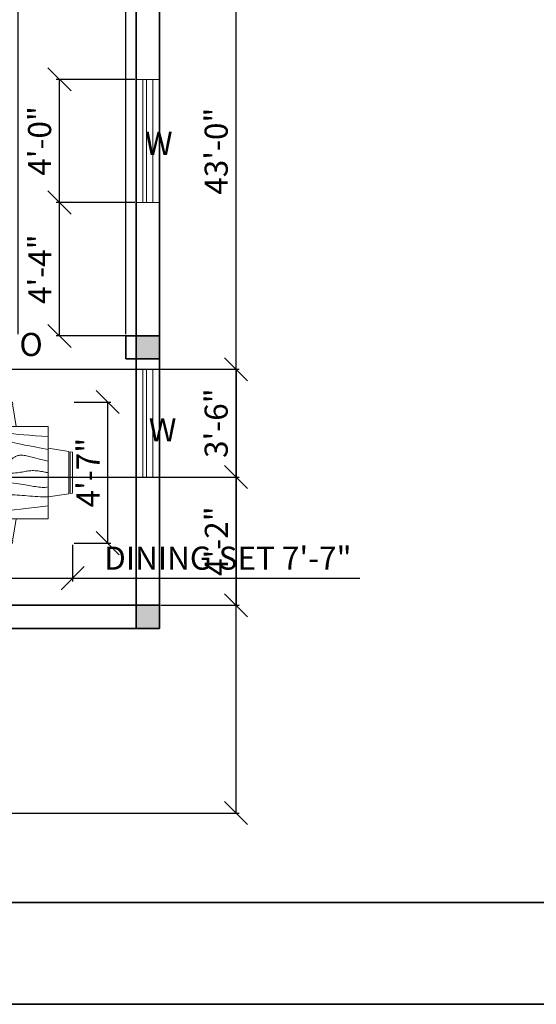
# Model space of a CAD drawing. Units: inches. Extents: x 1798 to 3594, y 1405 to 2404.
# Tile 3 of 6: x 2457 to 2658, y 1405 to 1789. Entities that reach past the tile are written whole.
import ezdxf

# ---------------------------------------------------------------- set-up
doc = ezdxf.new("R2010")
doc.units = ezdxf.units.IN
for name, color, linetype, lineweight in [('A-ANNO-DIMS', 6, 'Continuous', 18), ('A-ANNO-TEXT', 7, 'Continuous', 18), ('A-ANNO-TTLB', 7, 'Continuous', 35), ('A-FURN', 18, 'Continuous', 18), ('A-GLAZ', 4, 'Continuous', 18), ('A-WALL', 7, 'Continuous', 35), ('S-COLS', 1, 'Continuous', 35)]:
    doc.layers.add(name, color=color, linetype=linetype, lineweight=lineweight)
doc.styles.get("Standard").update_dxf_attribs({"font": 'arial.ttf'})
doc.dimstyles.new('ISO-25', dxfattribs={"dimtxt": 9, "dimasz": 9, "dimexe": 1.25, "dimexo": 0.625, "dimgap": 2, "dimtad": 1, "dimdec": 1, "dimlunit": 4, "dimtxsty": 'Standard', "dimblk": 'OBLIQUE', "dimcen": 2.5, "dimazin": 0, "dimtfac": 1, "dimtdec": 1, "dimtmove": 0, "dimatfit": 3, "dimfxl": 1, "dimarcsym": 0})

# ---------------------------------------------------------------- blocks, each defined once
blk = doc.blocks.new('Dining Set - 36 x 72 in.')
for p, q in [((-22, 27.5), (-22.1562, 26.50042)), ((-22, 27.5), (-6, 27.5)), ((-5.8437, 26.49966), (-6, 27.5)), ((6, 27.5), (5.8438, 26.50042)), ((6, 27.5), (22, 27.5)), ((22.1563, 26.49966), (22, 27.5)), ((-22.2343, 26.00059), (-23.4847, 17.99762)), ((-22.2304, 26), (-5.7608, 26)), ((-5.8416, 26.5), (-22.1534, 26.5)), ((-4.5152, 17.99762), (-5.7655, 25.99926)), ((5.7657, 26.00059), (4.5153, 17.99762)), ((5.7696, 26), (22.2392, 26)), ((22.1584, 26.5), (5.8466, 26.5)), ((23.4848, 17.99762), (22.2345, 25.99926)), ((36, 18), (-36, 18)), ((-36, 18), (-36, -18)), ((36, -18), (36, 18)), ((-45.5, 8), (-44.5004, 8.15617)), ((-45.5, 8), (-45.5, -8)), ((-44.5, -8.15843), (-44.5, 8.15338)), ((-44.0006, 8.23428), (-35.9976, 9.48474)), ((-44, 8.23041), (-44, -8.23915)), ((44.0006, 8.23428), (35.9976, 9.48474)), ((44, 8.23041), (44, -8.23915)), ((44.5, -8.15843), (44.5, 8.15338)), ((45.5, 8), (44.5005, 8.15617)), ((45.5, 8), (45.5, -8)), ((-44.4997, -8.15631), (-45.5, -8)), ((-35.9976, -9.48476), (-43.9993, -8.2345)), ((35.9976, -9.48476), (43.9993, -8.2345)), ((44.4997, -8.15631), (45.5, -8)), ((-36, -18), (36, -18)), ((-22.2343, -26.0006), (-23.4847, -17.99762)), ((-4.5152, -17.99762), (-5.7655, -25.99928)), ((5.7657, -26.0006), (4.5153, -17.99762)), ((23.4848, -17.99762), (22.2345, -25.99928)), ((-22.2304, -26), (-5.7608, -26)), ((-22, -27.5), (-22.1562, -26.50044)), ((-5.8416, -26.5), (-22.1534, -26.5)), ((-5.8437, -26.49967), (-6, -27.5)), ((5.7696, -26), (22.2392, -26)), ((6, -27.5), (5.8438, -26.50044)), ((22.1584, -26.5), (5.8466, -26.5)), ((22.1563, -26.49967), (22, -27.5)), ((-22, -27.5), (-6, -27.5)), ((6, -27.5), (22, -27.5))]:
    blk.add_line(p, q)
for points in [[(-36, 15), (-31.1772, 14.97754), (-26.8079, 14.91406), (-22.8538, 14.81543), (-19.276, 14.6875), (-16.0362, 14.53613), (-13.0957, 14.36718), (-10.4159, 14.18652), (-7.9583, 14), (-5.6904, 13.81315), (-3.6035, 13.63021), (-1.6954, 13.45508), (0.0365, 13.29166), (1.5945, 13.14388), (2.9811, 13.01562), (4.1988, 12.9108), (5.25, 12.83333), (6.1393, 12.78613), (6.8802, 12.76823), (7.4883, 12.77767), (7.9792, 12.8125), (8.3685, 12.87077), (8.6719, 12.95052), (8.9049, 13.0498), (9.0833, 13.16666), (9.2205, 13.29899), (9.3216, 13.44401), (9.3895, 13.59879), (9.4271, 13.76041), (9.4373, 13.92594), (9.4232, 14.09245), (9.3875, 14.257), (9.3333, 14.41666), (9.2638, 14.56917), (9.1836, 14.71484), (9.0975, 14.85465), (9.0104, 14.98958), (8.9272, 15.1206), (8.8529, 15.2487), (8.7922, 15.37483), (8.75, 15.5), (8.7305, 15.62467), (8.7344, 15.74739), (8.7617, 15.86621), (8.8125, 15.97916), (8.8867, 16.08431), (8.9844, 16.17968), (9.1055, 16.26334), (9.25, 16.33333), (9.4189, 16.38802), (9.6172, 16.42708), (9.8506, 16.45052), (10.125, 16.45833), (10.4463, 16.45052), (10.8203, 16.42708), (11.2529, 16.38802), (11.75, 16.33333), (12.3184, 16.26318), (12.9694, 16.17838), (13.7151, 16.07991), (14.5677, 15.96875), (15.5395, 15.84586), (16.6426, 15.71224), (17.8893, 15.56884), (19.2917, 15.41666), (20.859, 15.25667), (22.5879, 15.08984), (24.4721, 14.91715), (26.5052, 14.73958), (28.6809, 14.5581), (30.9929, 14.3737), (33.4347, 14.18733), (36, 14)], [(-36, 10), (-28.9766, 10.14274), (-23.1725, 10.20442), (-18.4241, 10.19775), (-14.5677, 10.13541), (-11.4399, 10.03011), (-8.877, 9.89453), (-6.7154, 9.74137), (-4.7917, 9.58333), (-2.9698, 9.43082), (-1.2246, 9.28515), (0.4415, 9.14534), (2.026, 9.01041), (3.5266, 8.87939), (4.9408, 8.7513), (6.266, 8.62516), (7.5, 8.5), (8.6411, 8.37549), (9.6914, 8.2539), (10.6538, 8.13818), (11.5312, 8.03125), (12.3267, 7.93603), (13.043, 7.85547), (13.6831, 7.79248), (14.25, 7.75), (14.7471, 7.7303), (15.1797, 7.73307), (15.5537, 7.75732), (15.875, 7.80208), (16.1494, 7.86637), (16.3828, 7.94922), (16.5811, 8.04964), (16.75, 8.16666), (16.8944, 8.29915), (17.0143, 8.44531), (17.1089, 8.60319), (17.1771, 8.77083), (17.218, 8.94629), (17.2305, 9.1276), (17.2137, 9.31282), (17.1667, 9.5), (17.0895, 9.6875), (16.987, 9.875), (16.8649, 10.0625), (16.7292, 10.25), (16.5856, 10.4375), (16.4401, 10.625), (16.2985, 10.8125), (16.1667, 11), (16.05, 11.18733), (15.9518, 11.3737), (15.8752, 11.5581), (15.8229, 11.73958), (15.798, 11.91715), (15.8034, 12.08984), (15.842, 12.25667), (15.9167, 12.41666), (16.0295, 12.56836), (16.1784, 12.70833), (16.3605, 12.83268), (16.5729, 12.9375), (16.8127, 13.01888), (17.0768, 13.07291), (17.3625, 13.0957), (17.6667, 13.08333), (17.9894, 13.03312), (18.3418, 12.94726), (18.7382, 12.82918), (19.1927, 12.68229), (19.7195, 12.51001), (20.3327, 12.31575), (21.0465, 12.10294), (21.875, 11.875), (22.8357, 11.63354), (23.959, 11.37304), (25.2786, 11.08618), (26.8282, 10.76562), (28.6414, 10.40405), (30.752, 9.99414), (33.1936, 9.52856), (36, 9)], [(-36, 5.5), (-30.7157, 5.3348), (-26.069, 5.20963), (-21.9946, 5.11767), (-18.4271, 5.05208), (-15.3009, 5.00602), (-12.5508, 4.97265), (-10.1112, 4.94515), (-7.9167, 4.91666), (-5.909, 4.88167), (-4.0586, 4.83984), (-2.3429, 4.79215), (-0.7396, 4.73958), (0.7739, 4.6831), (2.22, 4.6237), (3.6213, 4.56233), (5, 4.5), (6.373, 4.43782), (7.7344, 4.3776), (9.0723, 4.32129), (10.375, 4.27083), (11.6309, 4.22819), (12.8281, 4.19531), (13.9551, 4.17415), (15, 4.16666), (15.954, 4.17448), (16.819, 4.19791), (17.6001, 4.23698), (18.3021, 4.29166), (18.9299, 4.36198), (19.4883, 4.44791), (19.9823, 4.54948), (20.4167, 4.66666), (20.7969, 4.79899), (21.1302, 4.94401), (21.4245, 5.09879), (21.6875, 5.26041), (21.9271, 5.42594), (22.1511, 5.59245), (22.3672, 5.757), (22.5834, 5.91666), (22.8065, 6.06868), (23.0404, 6.21093), (23.2879, 6.34147), (23.5521, 6.45833), (23.8358, 6.55957), (24.142, 6.64323), (24.4735, 6.70735), (24.8334, 6.75), (25.2235, 6.76969), (25.642, 6.76692), (26.0858, 6.74267), (26.5521, 6.69791), (27.0379, 6.63362), (27.5404, 6.55078), (28.0565, 6.45036), (28.5834, 6.33333), (29.1242, 6.19987), (29.7071, 6.04687), (30.3661, 5.87044), (31.1354, 5.66666), (32.0493, 5.43164), (33.142, 5.16146), (34.4475, 4.85221), (36, 4.5)], [(-36, -1), (-30.7915, -0.6591), (-26.0195, -0.38216), (-21.6519, -0.16284), (-17.6563, 0.00521), (-14.0005, 0.12833), (-10.6523, 0.21289), (-7.5796, 0.26522), (-4.75, 0.29166), (-2.134, 0.29793), (0.2878, 0.28711), (2.5317, 0.26163), (4.6146, 0.22396), (6.5529, 0.17651), (8.3633, 0.12174), (10.0623, 0.06209), (11.6667, 0), (13.1899, -0.06201), (14.6341, -0.1211), (15.9982, -0.17432), (17.2813, -0.21875), (18.4823, -0.25147), (19.6003, -0.26953), (20.6343, -0.27002), (21.5834, -0.25), (22.4481, -0.20768), (23.2357, -0.14584), (23.9549, -0.06836), (24.6146, 0.02083), (25.2235, 0.11784), (25.7904, 0.21875), (26.3241, 0.31966), (26.8334, 0.41666), (27.3265, 0.50618), (27.8099, 0.58593), (28.2894, 0.65397), (28.7709, 0.70833), (29.2601, 0.74707), (29.763, 0.76823), (30.2855, 0.76985), (30.8334, 0.75), (31.4088, 0.70784), (31.9994, 0.64713), (32.589, 0.57275), (33.1615, 0.48958), (33.7008, 0.4025), (34.1908, 0.3164), (34.6153, 0.23616), (34.9584, 0.16666), (35.2099, 0.11165), (35.3848, 0.07031), (35.504, 0.04069), (35.5886, 0.02083), (35.6594, 0.00879), (35.7377, 0.0026), (35.8442, 0.00032), (36, 0)], [(-36, -6.5), (-27.1843, -6.31267), (-20.084, -6.1263), (-14.469, -5.9419), (-10.1094, -5.76042), (-6.7752, -5.58285), (-4.2363, -5.41016), (-2.2629, -5.24333), (-0.625, -5.08334), (0.8708, -4.93099), (2.2715, -4.78646), (3.5872, -4.64974), (4.8281, -4.52084), (6.0046, -4.39974), (7.127, -4.28646), (8.2053, -4.18099), (9.25, -4.08334), (10.2705, -3.99382), (11.2734, -3.91407), (12.2647, -3.84603), (13.25, -3.79167), (14.2354, -3.75293), (15.2266, -3.73177), (16.2295, -3.73015), (17.25, -3.75), (18.2912, -3.79248), (19.3451, -3.85547), (20.4009, -3.93604), (21.4479, -4.03125), (22.4754, -4.13819), (23.4727, -4.25391), (24.4289, -4.37549), (25.3334, -4.5), (26.1785, -4.62492), (26.9694, -4.74935), (27.7145, -4.87281), (28.4219, -4.99479), (29.1, -5.11483), (29.7572, -5.23242), (30.4016, -5.34709), (31.0417, -5.45834), (31.6837, -5.56437), (32.3262, -5.65821), (32.9658, -5.73153), (33.599, -5.77604), (34.2224, -5.78345), (34.8327, -5.74545), (35.4264, -5.65373), (36, -5.5)], [(-36, -10), (-26.4022, -9.81299), (-18.4675, -9.62891), (-11.9839, -9.45069), (-6.7396, -9.28125), (-2.5226, -9.12354), (0.8789, -8.98047), (3.6769, -8.85498), (6.0833, -8.75), (8.2767, -8.66765), (10.3021, -8.60677), (12.1712, -8.56543), (13.8958, -8.54167), (15.4876, -8.53353), (16.9583, -8.53907), (18.3197, -8.55632), (19.5834, -8.58334), (20.7616, -8.61841), (21.8685, -8.66081), (22.9188, -8.71004), (23.9271, -8.76563), (24.9081, -8.82707), (25.8763, -8.89388), (26.8465, -8.96558), (27.8334, -9.04167), (28.8474, -9.12118), (29.8828, -9.20117), (30.93, -9.27824), (31.9792, -9.34896), (33.0205, -9.40991), (34.0443, -9.45768), (35.0407, -9.48885), (36, -9.5)], [(-36, -14.5), (-30.0881, -14.33513), (-25.0332, -14.21224), (-20.7312, -14.12647), (-17.0781, -14.07292), (-13.97, -14.04671), (-11.3027, -14.04297), (-8.9724, -14.05681), (-6.875, -14.08334), (-4.9224, -14.11833), (-3.0905, -14.16016), (-1.3709, -14.20785), (0.2448, -14.26042), (1.7647, -14.3169), (3.1973, -14.3763), (4.5507, -14.43767), (5.8333, -14.5), (7.0554, -14.5621), (8.235, -14.62175), (9.3922, -14.67652), (10.5469, -14.72396), (11.7192, -14.76164), (12.929, -14.78711), (14.1965, -14.79794), (15.5417, -14.79167), (16.9933, -14.76424), (18.6152, -14.70508), (20.4804, -14.60197), (22.6615, -14.44271), (25.2312, -14.21509), (28.2624, -13.9069), (31.8277, -13.50594), (36, -13)]]:
    blk.add_lwpolyline(points)
blk = doc.blocks.new('COLUMN-9X9')
h = blk.add_hatch(color=256)
h.dxf.hatch_style = 1
h.paths.add_polyline_path([(9, 9), (0, 9), (0, 0), (9, 0)])
blk.add_lwpolyline([(0, 9), (9, 9), (9, 0), (0, 0)], close=True)
blk = doc.blocks.new('_Oblique')
at = {"color": 0, "linetype": 'ByBlock', "lineweight": -2}
blk.add_line((-0.5, -0.5), (0.5, 0.5), dxfattribs=at)
blk = doc.blocks.new('*D27')
at = {"layer": 'A-ANNO-DIMS', "color": 0, "lineweight": -2, "transparency": 16777216}
for p, q in [((2386.49, 1584.39), (2386.49, 1570.12)), ((2477.49, 1584.39), (2477.49, 1570.12)), ((2386.49, 1571.37), (2477.49, 1571.37)), ((2477.49, 1571.37), (2589.41, 1571.37))]:
    blk.add_line(p, q, dxfattribs=at)
at = {"layer": 'Defpoints', "color": 0, "transparency": 16777216}
for p in [(2386.49, 1585.02), (2477.49, 1585.02), (2477.49, 1571.37)]:
    blk.add_point(p, dxfattribs=at)
at = {"layer": 'A-ANNO-DIMS', "color": 0, "lineweight": -2, "transparency": 16777216, "xscale": 9, "yscale": 9, "zscale": 9, "rotation": 180}
blk.add_blockref('_Oblique', (2386.49, 1571.37), dxfattribs=at)
at = {"layer": 'A-ANNO-DIMS', "color": 0, "lineweight": -2, "transparency": 16777216, "xscale": 9, "yscale": 9, "zscale": 9}
blk.add_blockref('_Oblique', (2477.49, 1571.37), dxfattribs=at)
at = {"layer": 'A-ANNO-DIMS', "color": 0, "transparency": 16777216, "insert": (2537.95, 1578.02), "char_height": 9, "attachment_point": 5}
blk.add_mtext('DINING SET 7\'-7"', dxfattribs=at)
blk = doc.blocks.new('*D28')
at = {"layer": 'A-ANNO-DIMS', "color": 0, "lineweight": -2, "transparency": 16777216}
for p, q in [((2478.11, 1640.02), (2492.39, 1640.02)), ((2491.14, 1585.02), (2491.14, 1640.02)), ((2478.11, 1585.02), (2492.39, 1585.02))]:
    blk.add_line(p, q, dxfattribs=at)
at = {"layer": 'Defpoints', "color": 0, "transparency": 16777216}
for p in [(2477.49, 1640.02), (2491.14, 1640.02), (2477.49, 1585.02)]:
    blk.add_point(p, dxfattribs=at)
at = {"layer": 'A-ANNO-DIMS', "color": 0, "lineweight": -2, "transparency": 16777216, "xscale": 9, "yscale": 9, "zscale": 9}
for p, rotation in [((2491.14, 1640.02), 90), ((2491.14, 1585.02), 270)]:
    blk.add_blockref('_Oblique', p, dxfattribs=dict(at, rotation=rotation))
at = {"layer": 'A-ANNO-DIMS', "color": 0, "transparency": 16777216, "insert": (2484.64, 1612.52), "char_height": 9, "attachment_point": 5, "rotation": 90}
blk.add_mtext('4\'-7"', dxfattribs=at)
blk = doc.blocks.new('*D30')
at = {"layer": 'A-ANNO-DIMS', "color": 0, "lineweight": -2, "transparency": 16777216}
for p, q in [((2511.9, 1995.81), (2542.42, 1995.81)), ((2541.17, 1479.81), (2541.17, 1995.81)), ((2342.9, 1479.81), (2542.42, 1479.81))]:
    blk.add_line(p, q, dxfattribs=at)
at = {"layer": 'Defpoints', "color": 0, "transparency": 16777216}
for p in [(2511.27, 1995.81), (2541.17, 1995.81), (2342.27, 1479.81)]:
    blk.add_point(p, dxfattribs=at)
at = {"layer": 'A-ANNO-DIMS', "color": 0, "lineweight": -2, "transparency": 16777216, "xscale": 9, "yscale": 9, "zscale": 9}
for p, rotation in [((2541.17, 1995.81), 90), ((2541.17, 1479.81), 270)]:
    blk.add_blockref('_Oblique', p, dxfattribs=dict(at, rotation=rotation))
at = {"layer": 'A-ANNO-DIMS', "color": 0, "transparency": 16777216, "insert": (2534.57, 1737.81), "char_height": 9, "attachment_point": 5, "rotation": 90}
blk.add_mtext('43\'-0"', dxfattribs=at)
blk = doc.blocks.new('*D38')
at = {"layer": 'A-ANNO-DIMS', "color": 0, "lineweight": -2, "transparency": 16777216}
for p, q in [((2501.645352, 1717.811986), (2471.120352, 1717.811986)), ((2472.370352, 1665.811986), (2472.370352, 1717.811986)), ((2501.645352, 1665.811986), (2471.120352, 1665.811986))]:
    blk.add_line(p, q, dxfattribs=at)
at = {"layer": 'Defpoints', "color": 0, "transparency": 16777216}
for p in [(2472.370352, 1717.811986), (2502.270352, 1717.811986), (2502.270352, 1665.811986)]:
    blk.add_point(p, dxfattribs=at)
at = {"layer": 'A-ANNO-DIMS', "color": 0, "lineweight": -2, "transparency": 16777216, "xscale": 9, "yscale": 9, "zscale": 9}
for p, rotation in [((2472.370352, 1717.811986), 90), ((2472.370352, 1665.811986), 270)]:
    blk.add_blockref('_Oblique', p, dxfattribs=dict(at, rotation=rotation))
at = {"layer": 'A-ANNO-DIMS', "color": 0, "transparency": 16777216, "insert": (2465.870352, 1691.811986), "char_height": 9, "attachment_point": 5, "rotation": 90}
blk.add_mtext('4\'-4"', dxfattribs=at)
blk = doc.blocks.new('*D39')
at = {"layer": 'A-ANNO-DIMS', "color": 0, "lineweight": -2, "transparency": 16777216}
for p, q in [((2501.65, 1765.81), (2471.12, 1765.81)), ((2472.37, 1717.81), (2472.37, 1765.81)), ((2501.65, 1717.81), (2471.12, 1717.81))]:
    blk.add_line(p, q, dxfattribs=at)
at = {"layer": 'Defpoints', "color": 0, "transparency": 16777216}
for p in [(2472.37, 1765.81), (2502.27, 1765.81), (2502.27, 1717.81)]:
    blk.add_point(p, dxfattribs=at)
at = {"layer": 'A-ANNO-DIMS', "color": 0, "lineweight": -2, "transparency": 16777216, "xscale": 9, "yscale": 9, "zscale": 9}
for p, rotation in [((2472.37, 1765.81), 90), ((2472.37, 1717.81), 270)]:
    blk.add_blockref('_Oblique', p, dxfattribs=dict(at, rotation=rotation))
at = {"layer": 'A-ANNO-DIMS', "color": 0, "transparency": 16777216, "insert": (2465.78, 1741.81), "char_height": 9, "attachment_point": 5, "rotation": 90}
blk.add_mtext('4\'-0"', dxfattribs=at)
blk = doc.blocks.new('*D46')
at = {"layer": 'A-ANNO-DIMS', "color": 0, "lineweight": -2, "transparency": 16777216}
for p, q in [((2364.9, 1652.81), (2542.42, 1652.81)), ((2541.17, 1610.81), (2541.17, 1652.81)), ((2364.9, 1610.81), (2542.42, 1610.81))]:
    blk.add_line(p, q, dxfattribs=at)
at = {"layer": 'Defpoints', "color": 0, "transparency": 16777216}
for p in [(2364.27, 1652.81), (2541.17, 1652.81), (2364.27, 1610.81)]:
    blk.add_point(p, dxfattribs=at)
at = {"layer": 'A-ANNO-DIMS', "color": 0, "lineweight": -2, "transparency": 16777216, "xscale": 9, "yscale": 9, "zscale": 9}
for p, rotation in [((2541.17, 1652.81), 90), ((2541.17, 1610.81), 270)]:
    blk.add_blockref('_Oblique', p, dxfattribs=dict(at, rotation=rotation))
at = {"layer": 'A-ANNO-DIMS', "color": 0, "transparency": 16777216, "insert": (2534.57, 1631.81), "char_height": 9, "attachment_point": 5, "rotation": 90}
blk.add_mtext('3\'-6"', dxfattribs=at)
blk = doc.blocks.new('*D47')
at = {"layer": 'A-ANNO-DIMS', "color": 0, "lineweight": -2, "transparency": 16777216}
for p, q in [((2456.27, 1666.44), (2456.27, 2092.43)), ((2498.27, 1666.44), (2498.27, 2092.43)), ((2456.27, 2091.18), (2498.27, 2091.18))]:
    blk.add_line(p, q, dxfattribs=at)
at = {"layer": 'Defpoints', "color": 0, "transparency": 16777216}
for p in [(2498.27, 2091.18), (2456.27, 1665.81), (2498.27, 1665.81)]:
    blk.add_point(p, dxfattribs=at)
at = {"layer": 'A-ANNO-DIMS', "color": 0, "lineweight": -2, "transparency": 16777216, "xscale": 9, "yscale": 9, "zscale": 9, "rotation": 180}
blk.add_blockref('_Oblique', (2456.27, 2091.18), dxfattribs=at)
at = {"layer": 'A-ANNO-DIMS', "color": 0, "lineweight": -2, "transparency": 16777216, "xscale": 9, "yscale": 9, "zscale": 9}
blk.add_blockref('_Oblique', (2498.27, 2091.18), dxfattribs=at)
at = {"layer": 'A-ANNO-DIMS', "color": 0, "transparency": 16777216, "insert": (2477.27, 2097.78), "char_height": 9, "attachment_point": 5}
blk.add_mtext('3\'-6"', dxfattribs=at)
blk = doc.blocks.new('*D49')
at = {"layer": 'A-ANNO-DIMS', "color": 0, "lineweight": -2, "transparency": 16777216}
for p, q in [((2511.9, 1652.81), (2542.42, 1652.81)), ((2541.17, 1652.81), (2541.17, 1610.81)), ((2511.9, 1610.81), (2542.42, 1610.81))]:
    blk.add_line(p, q, dxfattribs=at)
at = {"layer": 'Defpoints', "color": 0, "transparency": 16777216}
for p in [(2511.27, 1652.81), (2511.27, 1610.81), (2541.17, 1610.81)]:
    blk.add_point(p, dxfattribs=at)
at = {"layer": 'A-ANNO-DIMS', "color": 0, "lineweight": -2, "transparency": 16777216, "xscale": 9, "yscale": 9, "zscale": 9}
for p, rotation in [((2541.17, 1652.81), 90), ((2541.17, 1610.81), 270)]:
    blk.add_blockref('_Oblique', p, dxfattribs=dict(at, rotation=rotation))
at = {"layer": 'A-ANNO-DIMS', "color": 0, "transparency": 16777216, "insert": (2534.57, 1631.81), "char_height": 9, "attachment_point": 5, "rotation": 90}
blk.add_mtext('3\'-6"', dxfattribs=at)
blk = doc.blocks.new('*D50')
at = {"layer": 'A-ANNO-DIMS', "color": 0, "lineweight": -2, "transparency": 16777216}
for p, q in [((2511.9, 1610.81), (2542.42, 1610.81)), ((2541.17, 1610.81), (2541.17, 1560.81)), ((2511.9, 1560.81), (2542.42, 1560.81))]:
    blk.add_line(p, q, dxfattribs=at)
at = {"layer": 'Defpoints', "color": 0, "transparency": 16777216}
for p in [(2511.27, 1610.81), (2511.27, 1560.81), (2541.17, 1560.81)]:
    blk.add_point(p, dxfattribs=at)
at = {"layer": 'A-ANNO-DIMS', "color": 0, "lineweight": -2, "transparency": 16777216, "xscale": 9, "yscale": 9, "zscale": 9}
for p, rotation in [((2541.17, 1610.81), 90), ((2541.17, 1560.81), 270)]:
    blk.add_blockref('_Oblique', p, dxfattribs=dict(at, rotation=rotation))
at = {"layer": 'A-ANNO-DIMS', "color": 0, "transparency": 16777216, "insert": (2534.65, 1585.81), "char_height": 9, "attachment_point": 5, "rotation": 90}
blk.add_mtext('4\'-2"', dxfattribs=at)

msp = doc.modelspace()

# ---------------------------------------------------------------- linework, layer by layer
at = {"layer": 'A-ANNO-TTLB'}
for points in [[(1798.35, 2403.73), (3594.23, 2403.73), (3594.23, 1405.28), (1798.35, 1405.28)], [(1855.68, 2366.05), (3540.6, 2366.05), (3540.6, 1444.98), (1855.68, 1444.98)]]:
    msp.add_lwpolyline(points, close=True, dxfattribs=at)
at = {"layer": 'A-GLAZ'}
for p, q in [((2502.27, 1765.81), (2511.27, 1765.81)), ((2504.77, 1765.81), (2504.77, 1717.81)), ((2506.27, 1765.81), (2506.27, 1717.81)), ((2508.77, 1765.81), (2508.77, 1717.81)), ((2502.27, 1717.81), (2511.27, 1717.81)), ((2502.27, 1652.81), (2511.27, 1652.81)), ((2502.27, 1652.81), (2511.27, 1652.81)), ((2504.77, 1652.81), (2504.77, 1610.81)), ((2506.27, 1652.81), (2506.27, 1610.81)), ((2508.77, 1652.81), (2508.77, 1610.81)), ((2502.27, 1610.81), (2511.27, 1610.81))]:
    msp.add_line(p, q, dxfattribs=at)
at = {"layer": 'A-WALL'}
for p, q in [((2511.27, 1995.81), (2511.27, 1551.81)), ((2502.27, 1857.81), (2502.27, 1551.81)), ((2498.27, 1665.81), (2498.27, 1656.81)), ((2498.27, 1665.81), (2511.27, 1665.81)), ((2498.27, 1656.81), (2511.27, 1656.81)), ((2226.27, 1560.81), (2511.27, 1560.81)), ((2226.27, 1551.81), (2511.27, 1551.81))]:
    msp.add_line(p, q, dxfattribs=at)

# ---------------------------------------------------------------- block references
at = {"layer": 'A-FURN'}
msp.add_blockref('Dining Set - 36 x 72 in.', (2431.99, 1612.52), dxfattribs=at)
at = {"layer": 'S-COLS'}
for p in [(2502.27, 1656.81), (2502.27, 1551.81)]:
    msp.add_blockref('COLUMN-9X9', p, dxfattribs=at)

# ---------------------------------------------------------------- texts
at = {"layer": 'A-ANNO-TEXT'}
for s, p in [('               W', (2464.4, 1736.38)), ('               O', (2415.48, 1657.97)), ('               W', (2465.89, 1624.68))]:
    msp.add_text(s, height=9, dxfattribs=at).set_placement(p)

# ---------------------------------------------------------------- dimensions: what is measured, and where the dimension line sits
at = {"layer": 'A-ANNO-DIMS'}
dim = msp.add_linear_dim(base=(2498.27, 2091.18), p1=(2456.27, 1665.81), p2=(2498.27, 1665.81), dimstyle='ISO-25', override={"dimdec": 1, "dimlfac": 1, "dimrnd": 0, "dimzin": 1, "dimdsep": 46, "dimlunit": 4, "dimfrac": 2}, dxfattribs=at)
dim.commit()
dim.dimension.update_dxf_attribs({"geometry": '*D47', "text_midpoint": (2477.27, 2097.78)})
for base, p1, p2, angle, picture, middle in [((2541.17, 1995.81), (2342.27, 1479.81), (2511.27, 1995.81), 90, '*D30', (2534.57, 1737.81)), ((2472.37, 1765.81), (2502.27, 1717.81), (2502.27, 1765.81), 90, '*D39', (2465.78, 1741.81)), ((2472.37, 1717.81), (2502.27, 1665.81), (2502.27, 1717.81), 90, '*D38', (2465.87, 1691.81)), ((2541.17, 1652.81), (2364.27, 1610.81), (2364.27, 1652.81), 90, '*D46', (2534.57, 1631.81)), ((2541.17, 1610.81), (2511.27, 1652.81), (2511.27, 1610.81), 270, '*D49', (2534.57, 1631.81)), ((2491.14, 1640.02), (2477.49, 1585.02), (2477.49, 1640.02), 90, '*D28', (2484.64, 1612.52)), ((2541.17, 1560.81), (2511.27, 1610.81), (2511.27, 1560.81), 270, '*D50', (2534.65, 1585.81))]:
    dim = msp.add_linear_dim(base=base, p1=p1, p2=p2, angle=angle, dimstyle='ISO-25', override={"dimdec": 1, "dimlfac": 1, "dimrnd": 0, "dimzin": 1, "dimdsep": 46, "dimlunit": 4, "dimfrac": 2}, dxfattribs=at)
    dim.commit()
    dim.dimension.update_dxf_attribs({"geometry": picture, "text_midpoint": middle})
dim = msp.add_linear_dim(base=(2477.49, 1571.37), p1=(2386.49, 1585.02), p2=(2477.49, 1585.02), text='DINING SET <>', dimstyle='ISO-25', override={"dimdec": 1, "dimlfac": 1, "dimrnd": 0, "dimzin": 1, "dimdsep": 46, "dimlunit": 4, "dimfrac": 2}, dxfattribs=at)
dim.commit()
dim.dimension.update_dxf_attribs({"geometry": '*D27', "text_midpoint": (2537.95, 1578.02)})

doc.saveas('drawing.dxf')
